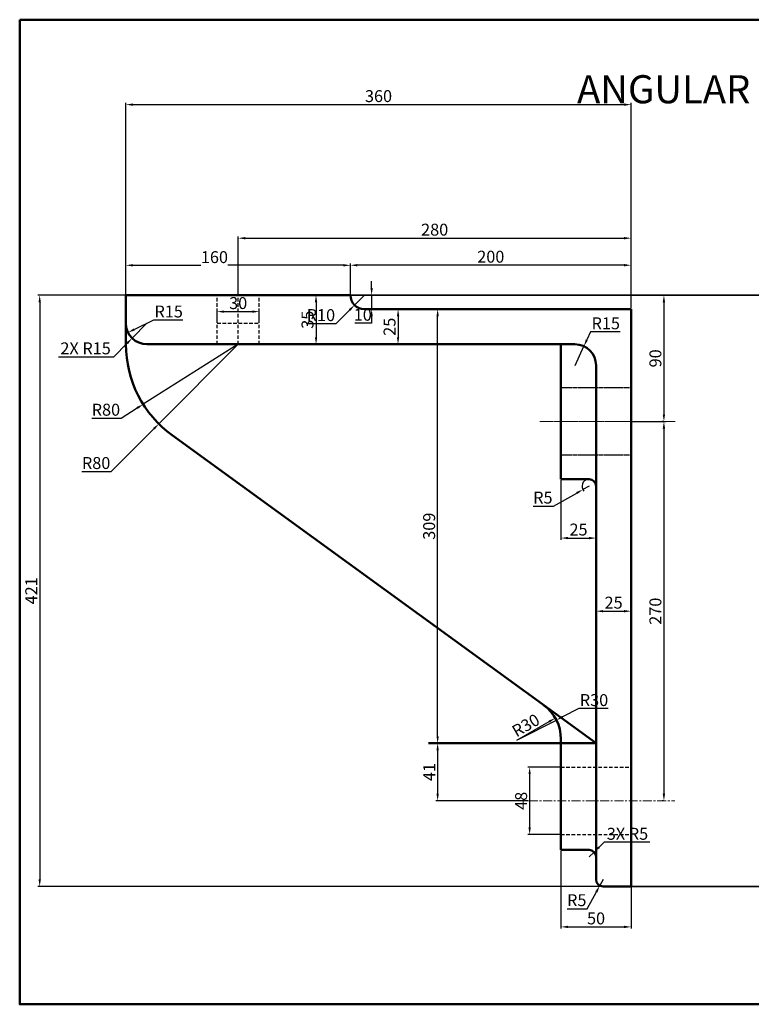
# Model space of a CAD drawing. Units: millimetres. Extents: x -624 to 605, y 670 to 1371.
# Tile 1 of 2: x -624 to -102, y 670 to 1371. Entities that reach past the tile are written whole.
import ezdxf

# ---------------------------------------------------------------- set-up
doc = ezdxf.new("R2010")
doc.units = ezdxf.units.MM
doc.header["$LTSCALE"] = 0.2
doc.linetypes.add('CENTER', pattern=[50.8, 31.75, -6.35, 6.35, -6.35])
doc.linetypes.add('DASHED', pattern=[19.05, 12.7, -6.35])
for name, color, linetype, lineweight in [('M-CNTR', 1, 'CENTER', 18), ('M-DIMS', 2, 'Continuous', 25), ('M-HIDN', 4, 'DASHED', 25), ('M-OUTL', 7, 'Continuous', 50), ('M-TEXT', 7, 'Continuous', 25)]:
    doc.layers.add(name, color=color, linetype=linetype, lineweight=lineweight)
doc.styles.get("Standard").update_dxf_attribs({"font": 'arial.ttf'})
doc.dimstyles.new('ISO-25', dxfattribs={"dimtxt": 8.5, "dimasz": 5, "dimexe": 1.25, "dimexo": 0.625, "dimtad": 1, "dimtoh": 1, "dimtxsty": 'Standard', "dimcen": 2.5, "dimadec": 0, "dimazin": 0, "dimtfac": 1, "dimtmove": 0, "dimatfit": 3, "dimfxl": 1, "dimarcsym": 0})

# ---------------------------------------------------------------- blocks, each defined once
blk = doc.blocks.new('*D1')
at = {"layer": 'Defpoints', "color": 0, "ltscale": 0.2, "transparency": 16777216}
for p in [(-354.19, 1164.58), (-354.19, 1139.58), (-354.19, 1139.58)]:
    blk.add_point(p, dxfattribs=at)
at = {"layer": 'M-DIMS', "color": 0, "lineweight": -2, "ltscale": 0.2, "transparency": 16777216}
for p, q in [((-354.82, 1164.58), (-355.44, 1164.58)), ((-354.19, 1159.58), (-354.19, 1144.58)), ((-354.82, 1139.58), (-355.44, 1139.58))]:
    blk.add_line(p, q, dxfattribs=at)
at = {"layer": 'M-DIMS', "color": 0, "ltscale": 0.2, "transparency": 16777216}
for points in [[(-355.03, 1159.58), (-353.36, 1159.58), (-354.19, 1164.58)], [(-355.03, 1144.58), (-353.36, 1144.58), (-354.19, 1139.58)]]:
    blk.add_solid(points, dxfattribs=at)
at = {"layer": 'M-DIMS', "color": 0, "ltscale": 0.2, "transparency": 16777216, "insert": (-359.16, 1152.08), "char_height": 8.5, "attachment_point": 5, "rotation": 90}
blk.add_mtext('25', dxfattribs=at)
blk = doc.blocks.new('*D2')
at = {"layer": 'Defpoints', "color": 0, "ltscale": 0.2, "transparency": 16777216}
for p in [(-548.12, 1195.84), (-548.12, 1174.58), (-388.12, 1174.58)]:
    blk.add_point(p, dxfattribs=at)
at = {"layer": 'M-DIMS', "color": 0, "lineweight": -2, "ltscale": 0.2, "transparency": 16777216}
for p, q in [((-548.12, 1175.21), (-548.12, 1197.09)), ((-543.12, 1195.84), (-494.63, 1195.84)), ((-393.12, 1195.84), (-475.43, 1195.84)), ((-388.12, 1175.21), (-388.12, 1197.09))]:
    blk.add_line(p, q, dxfattribs=at)
at = {"layer": 'M-DIMS', "color": 0, "ltscale": 0.2, "transparency": 16777216}
for points in [[(-543.12, 1196.68), (-543.12, 1195.01), (-548.12, 1195.84)], [(-393.12, 1196.68), (-393.12, 1195.01), (-388.12, 1195.84)]]:
    blk.add_solid(points, dxfattribs=at)
at = {"layer": 'M-DIMS', "color": 0, "ltscale": 0.2, "transparency": 16777216, "insert": (-485.03, 1200.55), "char_height": 8.5, "attachment_point": 5}
blk.add_mtext('160', dxfattribs=at)
blk = doc.blocks.new('*D3')
at = {"layer": 'Defpoints', "color": 0, "ltscale": 0.2, "transparency": 16777216}
for p in [(-388.12, 1174.58), (-373.46, 1164.58), (-373.03, 1164.58)]:
    blk.add_point(p, dxfattribs=at)
at = {"layer": 'M-DIMS', "color": 0, "lineweight": -2, "ltscale": 0.2, "transparency": 16777216}
for p, q in [((-373.03, 1179.58), (-373.03, 1184.58)), ((-387.5, 1174.58), (-371.78, 1174.58)), ((-373.03, 1174.58), (-373.03, 1164.58)), ((-372.83, 1164.58), (-371.78, 1164.58)), ((-373.03, 1159.58), (-373.03, 1154.58)), ((-373.03, 1154.58), (-385, 1154.58))]:
    blk.add_line(p, q, dxfattribs=at)
at = {"layer": 'M-DIMS', "color": 0, "ltscale": 0.2, "transparency": 16777216}
for points in [[(-373.87, 1179.58), (-372.2, 1179.58), (-373.03, 1174.58)], [(-373.87, 1159.58), (-372.2, 1159.58), (-373.03, 1164.58)]]:
    blk.add_solid(points, dxfattribs=at)
at = {"layer": 'M-DIMS', "color": 0, "ltscale": 0.2, "transparency": 16777216, "insert": (-379.33, 1159.55), "char_height": 8.5, "attachment_point": 5}
blk.add_mtext('10', dxfattribs=at)
blk = doc.blocks.new('*D4')
at = {"layer": 'Defpoints', "color": 0, "ltscale": 0.2, "transparency": 16777216}
for p in [(-388.12, 1195.89), (-388.12, 1174.58), (-188.12, 1164.58)]:
    blk.add_point(p, dxfattribs=at)
at = {"layer": 'M-DIMS', "color": 0, "lineweight": -2, "ltscale": 0.2, "transparency": 16777216}
for p, q in [((-388.12, 1175.21), (-388.12, 1197.14)), ((-193.12, 1195.89), (-383.12, 1195.89)), ((-188.12, 1165.21), (-188.12, 1197.14))]:
    blk.add_line(p, q, dxfattribs=at)
at = {"layer": 'M-DIMS', "color": 0, "ltscale": 0.2, "transparency": 16777216}
for points in [[(-383.12, 1196.73), (-383.12, 1195.06), (-388.12, 1195.89)], [(-193.12, 1196.73), (-193.12, 1195.06), (-188.12, 1195.89)]]:
    blk.add_solid(points, dxfattribs=at)
at = {"layer": 'M-DIMS', "color": 0, "ltscale": 0.2, "transparency": 16777216, "insert": (-288.12, 1200.86), "char_height": 8.5, "attachment_point": 5}
blk.add_mtext('200', dxfattribs=at)
blk = doc.blocks.new('*D5')
at = {"layer": 'Defpoints', "color": 0, "ltscale": 0.2, "transparency": 16777216}
for p in [(-453.12, 1162.86), (-483.12, 1154.58), (-453.12, 1154.58)]:
    blk.add_point(p, dxfattribs=at)
at = {"layer": 'M-DIMS', "color": 0, "lineweight": -2, "ltscale": 0.2, "transparency": 16777216}
for p, q in [((-483.12, 1155.21), (-483.12, 1164.11)), ((-453.12, 1155.21), (-453.12, 1164.11)), ((-478.12, 1162.86), (-458.12, 1162.86))]:
    blk.add_line(p, q, dxfattribs=at)
at = {"layer": 'M-DIMS', "color": 0, "ltscale": 0.2, "transparency": 16777216}
for points in [[(-478.12, 1163.69), (-478.12, 1162.03), (-483.12, 1162.86)], [(-458.12, 1163.69), (-458.12, 1162.03), (-453.12, 1162.86)]]:
    blk.add_solid(points, dxfattribs=at)
at = {"layer": 'M-DIMS', "color": 0, "ltscale": 0.2, "transparency": 16777216, "insert": (-468.12, 1167.83), "char_height": 8.5, "attachment_point": 5}
blk.add_mtext('30', dxfattribs=at)
blk = doc.blocks.new('*D6')
at = {"layer": 'Defpoints', "color": 0, "ltscale": 0.2, "transparency": 16777216}
for p in [(-410.05, 1174.58), (-412.64, 1139.58), (-410.05, 1139.58)]:
    blk.add_point(p, dxfattribs=at)
at = {"layer": 'M-DIMS', "color": 0, "lineweight": -2, "ltscale": 0.2, "transparency": 16777216}
for p, q in [((-410.68, 1174.58), (-413.89, 1174.58)), ((-412.64, 1169.58), (-412.64, 1144.58)), ((-410.68, 1139.58), (-413.89, 1139.58))]:
    blk.add_line(p, q, dxfattribs=at)
at = {"layer": 'M-DIMS', "color": 0, "ltscale": 0.2, "transparency": 16777216}
for points in [[(-413.47, 1169.58), (-411.81, 1169.58), (-412.64, 1174.58)], [(-413.47, 1144.58), (-411.81, 1144.58), (-412.64, 1139.58)]]:
    blk.add_solid(points, dxfattribs=at)
at = {"layer": 'M-DIMS', "color": 0, "ltscale": 0.2, "transparency": 16777216, "insert": (-417.61, 1157.08), "char_height": 8.5, "attachment_point": 5, "rotation": 90}
blk.add_mtext('35', dxfattribs=at)
blk = doc.blocks.new('*D7')
at = {"layer": 'Defpoints', "color": 0, "ltscale": 0.2, "transparency": 16777216}
for p in [(-188.12, 1215.14), (-468.12, 1174.58), (-188.12, 1164.58)]:
    blk.add_point(p, dxfattribs=at)
at = {"layer": 'M-DIMS', "color": 0, "lineweight": -2, "ltscale": 0.2, "transparency": 16777216}
for p, q in [((-468.12, 1175.21), (-468.12, 1216.39)), ((-463.12, 1215.14), (-193.12, 1215.14)), ((-188.12, 1165.21), (-188.12, 1216.39))]:
    blk.add_line(p, q, dxfattribs=at)
at = {"layer": 'M-DIMS', "color": 0, "ltscale": 0.2, "transparency": 16777216}
for points in [[(-463.12, 1215.97), (-463.12, 1214.31), (-468.12, 1215.14)], [(-193.12, 1215.97), (-193.12, 1214.31), (-188.12, 1215.14)]]:
    blk.add_solid(points, dxfattribs=at)
at = {"layer": 'M-DIMS', "color": 0, "ltscale": 0.2, "transparency": 16777216, "insert": (-328.12, 1220.11), "char_height": 8.5, "attachment_point": 5}
blk.add_mtext('280', dxfattribs=at)
blk = doc.blocks.new('*D8')
at = {"layer": 'Defpoints', "color": 0, "ltscale": 0.2, "transparency": 16777216}
for p in [(-533.12, 1154.58), (-546.59, 1147.98)]:
    blk.add_point(p, dxfattribs=at)
at = {"layer": 'M-DIMS', "color": 0, "lineweight": -2, "ltscale": 0.2, "transparency": 16777216}
for p, q in [((-528.44, 1156.87), (-542.1, 1150.18)), ((-507.44, 1156.87), (-528.44, 1156.87))]:
    blk.add_line(p, q, dxfattribs=at)
at = {"layer": 'M-DIMS', "color": 0, "ltscale": 0.2, "transparency": 16777216}
blk.add_solid([(-542.47, 1150.93), (-541.74, 1149.43), (-546.59, 1147.98)], dxfattribs=at)
at = {"layer": 'M-DIMS', "color": 0, "ltscale": 0.2, "transparency": 16777216, "insert": (-517.63, 1161.84), "char_height": 8.5, "attachment_point": 5}
blk.add_mtext('R15', dxfattribs=at)
blk = doc.blocks.new('*D9')
at = {"layer": 'Defpoints', "color": 0, "ltscale": 0.2, "transparency": 16777216}
for p in [(-468.12, 1139.58), (-535.79, 1096.91)]:
    blk.add_point(p, dxfattribs=at)
at = {"layer": 'M-DIMS', "color": 0, "lineweight": -2, "ltscale": 0.2, "transparency": 16777216}
for p, q in [((-468.12, 1139.58), (-535.79, 1096.91)), ((-551.59, 1086.95), (-540.02, 1094.24)), ((-572.5, 1086.95), (-551.59, 1086.95))]:
    blk.add_line(p, q, dxfattribs=at)
at = {"layer": 'M-DIMS', "color": 0, "ltscale": 0.2, "transparency": 16777216}
blk.add_solid([(-540.47, 1094.95), (-539.58, 1093.54), (-535.79, 1096.91)], dxfattribs=at)
at = {"layer": 'M-DIMS', "color": 0, "ltscale": 0.2, "transparency": 16777216, "insert": (-562.36, 1091.91), "char_height": 8.5, "attachment_point": 5}
blk.add_mtext('R80', dxfattribs=at)
blk = doc.blocks.new('*D10')
at = {"layer": 'Defpoints', "color": 0, "ltscale": 0.2, "transparency": 16777216}
for p in [(-326.01, 1164.58), (-305.32, 1164.58), (-305.32, 855.58)]:
    blk.add_point(p, dxfattribs=at)
at = {"layer": 'M-DIMS', "color": 0, "lineweight": -2, "ltscale": 0.2, "transparency": 16777216}
for p, q in [((-305.94, 1164.58), (-327.26, 1164.58)), ((-326.01, 860.58), (-326.01, 1159.58)), ((-305.94, 855.58), (-327.26, 855.58))]:
    blk.add_line(p, q, dxfattribs=at)
at = {"layer": 'M-DIMS', "color": 0, "ltscale": 0.2, "transparency": 16777216}
for points in [[(-326.84, 1159.58), (-325.17, 1159.58), (-326.01, 1164.58)], [(-326.84, 860.58), (-325.17, 860.58), (-326.01, 855.58)]]:
    blk.add_solid(points, dxfattribs=at)
at = {"layer": 'M-DIMS', "color": 0, "ltscale": 0.2, "transparency": 16777216, "insert": (-330.97, 1010.08), "char_height": 8.5, "attachment_point": 5, "rotation": 90}
blk.add_mtext('309', dxfattribs=at)
blk = doc.blocks.new('*D11')
at = {"layer": 'Defpoints', "color": 0, "ltscale": 0.2, "transparency": 16777216}
for p in [(-316.6, 855.58), (-326.01, 814.58), (-260.98, 814.58)]:
    blk.add_point(p, dxfattribs=at)
at = {"layer": 'M-DIMS', "color": 0, "lineweight": -2, "ltscale": 0.2, "transparency": 16777216}
for p, q in [((-317.22, 855.58), (-327.26, 855.58)), ((-326.01, 850.58), (-326.01, 819.58)), ((-261.61, 814.58), (-327.26, 814.58))]:
    blk.add_line(p, q, dxfattribs=at)
at = {"layer": 'M-DIMS', "color": 0, "ltscale": 0.2, "transparency": 16777216}
for points in [[(-326.84, 850.58), (-325.17, 850.58), (-326.01, 855.58)], [(-326.84, 819.58), (-325.17, 819.58), (-326.01, 814.58)]]:
    blk.add_solid(points, dxfattribs=at)
at = {"layer": 'M-DIMS', "color": 0, "ltscale": 0.2, "transparency": 16777216, "insert": (-330.9, 835.08), "char_height": 8.5, "attachment_point": 5, "rotation": 90}
blk.add_mtext('41', dxfattribs=at)
blk = doc.blocks.new('*D12')
at = {"layer": 'Defpoints', "color": 0, "ltscale": 0.2, "transparency": 16777216}
for p in [(-238.12, 838.58), (-260.44, 790.58), (-238.12, 790.58)]:
    blk.add_point(p, dxfattribs=at)
at = {"layer": 'M-DIMS', "color": 0, "lineweight": -2, "ltscale": 0.2, "transparency": 16777216}
for p, q in [((-238.75, 838.58), (-261.69, 838.58)), ((-260.44, 833.58), (-260.44, 795.58)), ((-238.75, 790.58), (-261.69, 790.58))]:
    blk.add_line(p, q, dxfattribs=at)
at = {"layer": 'M-DIMS', "color": 0, "ltscale": 0.2, "transparency": 16777216}
for points in [[(-261.28, 833.58), (-259.61, 833.58), (-260.44, 838.58)], [(-261.28, 795.58), (-259.61, 795.58), (-260.44, 790.58)]]:
    blk.add_solid(points, dxfattribs=at)
at = {"layer": 'M-DIMS', "color": 0, "ltscale": 0.2, "transparency": 16777216, "insert": (-265.41, 814.58), "char_height": 8.5, "attachment_point": 5, "rotation": 90}
blk.add_mtext('48', dxfattribs=at)
blk = doc.blocks.new('*D13')
at = {"layer": 'Defpoints', "color": 0, "ltscale": 0.2, "transparency": 16777216}
for p in [(-242.17, 873.48), (-268.12, 858.44)]:
    blk.add_point(p, dxfattribs=at)
at = {"layer": 'M-DIMS', "color": 0, "lineweight": -2, "ltscale": 0.2, "transparency": 16777216}
blk.add_line((-269.45, 857.67), (-246.49, 870.97), dxfattribs=at)
at = {"layer": 'M-DIMS', "color": 0, "ltscale": 0.2, "transparency": 16777216}
blk.add_solid([(-246.91, 871.7), (-246.08, 870.25), (-242.17, 873.48)], dxfattribs=at)
at = {"layer": 'M-DIMS', "color": 0, "ltscale": 0.2, "transparency": 16777216, "insert": (-262.63, 867.37), "char_height": 8.5, "attachment_point": 5, "rotation": 30.09395}
blk.add_mtext('R30', dxfattribs=at)
blk = doc.blocks.new('*D14')
at = {"layer": 'Defpoints', "color": 0, "ltscale": 0.2, "transparency": 16777216}
for p in [(-238.12, 779.58), (-188.12, 779.58), (-188.12, 724.81)]:
    blk.add_point(p, dxfattribs=at)
at = {"layer": 'M-DIMS', "color": 0, "lineweight": -2, "ltscale": 0.2, "transparency": 16777216}
for p, q in [((-238.12, 778.96), (-238.12, 723.56)), ((-188.12, 778.96), (-188.12, 723.56)), ((-233.12, 724.81), (-193.12, 724.81))]:
    blk.add_line(p, q, dxfattribs=at)
at = {"layer": 'M-DIMS', "color": 0, "ltscale": 0.2, "transparency": 16777216}
for points in [[(-233.12, 725.64), (-233.12, 723.97), (-238.12, 724.81)], [(-193.12, 725.64), (-193.12, 723.97), (-188.12, 724.81)]]:
    blk.add_solid(points, dxfattribs=at)
at = {"layer": 'M-DIMS', "color": 0, "ltscale": 0.2, "transparency": 16777216, "insert": (-213.12, 729.77), "char_height": 8.5, "attachment_point": 5}
blk.add_mtext('50', dxfattribs=at)
blk = doc.blocks.new('*D15')
at = {"layer": 'Defpoints', "color": 0, "ltscale": 0.2, "transparency": 16777216}
for p in [(-208.12, 758.58), (-210.5, 754.18)]:
    blk.add_point(p, dxfattribs=at)
at = {"layer": 'M-DIMS', "color": 0, "lineweight": -2, "ltscale": 0.2, "transparency": 16777216}
for p, q in [((-208.12, 758.58), (-210.5, 754.18)), ((-219.36, 737.77), (-212.88, 749.78)), ((-233.75, 737.77), (-219.36, 737.77))]:
    blk.add_line(p, q, dxfattribs=at)
at = {"layer": 'M-DIMS', "color": 0, "ltscale": 0.2, "transparency": 16777216}
blk.add_solid([(-213.61, 750.18), (-212.14, 749.39), (-210.5, 754.18)], dxfattribs=at)
at = {"layer": 'M-DIMS', "color": 0, "ltscale": 0.2, "transparency": 16777216, "insert": (-226.87, 742.72), "char_height": 8.5, "attachment_point": 5}
blk.add_mtext('R5', dxfattribs=at)
blk = doc.blocks.new('*D16')
at = {"layer": 'Defpoints', "color": 0, "ltscale": 0.2, "transparency": 16777216}
for p in [(-213.12, 949.58), (-188.12, 949.58), (-188.12, 949.58)]:
    blk.add_point(p, dxfattribs=at)
at = {"layer": 'M-DIMS', "color": 0, "lineweight": -2, "ltscale": 0.2, "transparency": 16777216}
for p, q in [((-213.12, 950.21), (-213.12, 950.83)), ((-208.12, 949.58), (-193.12, 949.58)), ((-188.12, 950.21), (-188.12, 950.83))]:
    blk.add_line(p, q, dxfattribs=at)
at = {"layer": 'M-DIMS', "color": 0, "ltscale": 0.2, "transparency": 16777216}
for points in [[(-208.12, 950.41), (-208.12, 948.75), (-213.12, 949.58)], [(-193.12, 950.41), (-193.12, 948.75), (-188.12, 949.58)]]:
    blk.add_solid(points, dxfattribs=at)
at = {"layer": 'M-DIMS', "color": 0, "ltscale": 0.2, "transparency": 16777216, "insert": (-200.62, 954.55), "char_height": 8.5, "attachment_point": 5}
blk.add_mtext('25', dxfattribs=at)
blk = doc.blocks.new('*D17')
at = {"layer": 'Defpoints', "color": 0, "ltscale": 0.2, "transparency": 16777216}
for p in [(-388.12, 1174.58), (-188.12, 1084.58), (-164.76, 1084.58)]:
    blk.add_point(p, dxfattribs=at)
at = {"layer": 'M-DIMS', "color": 0, "lineweight": -2, "ltscale": 0.2, "transparency": 16777216}
for p, q in [((-387.5, 1174.58), (-163.51, 1174.58)), ((-164.76, 1169.58), (-164.76, 1089.58)), ((-187.5, 1084.58), (-163.51, 1084.58))]:
    blk.add_line(p, q, dxfattribs=at)
at = {"layer": 'M-DIMS', "color": 0, "ltscale": 0.2, "transparency": 16777216}
for points in [[(-165.6, 1169.58), (-163.93, 1169.58), (-164.76, 1174.58)], [(-165.6, 1089.58), (-163.93, 1089.58), (-164.76, 1084.58)]]:
    blk.add_solid(points, dxfattribs=at)
at = {"layer": 'M-DIMS', "color": 0, "ltscale": 0.2, "transparency": 16777216, "insert": (-169.73, 1129.58), "char_height": 8.5, "attachment_point": 5, "rotation": 90}
blk.add_mtext('90', dxfattribs=at)
blk = doc.blocks.new('*D18')
at = {"layer": 'Defpoints', "color": 0, "ltscale": 0.2, "transparency": 16777216}
for p in [(-164.76, 1084.58), (-164.76, 814.58), (-164.76, 814.58)]:
    blk.add_point(p, dxfattribs=at)
at = {"layer": 'M-DIMS', "color": 0, "lineweight": -2, "ltscale": 0.2, "transparency": 16777216}
for p, q in [((-165.39, 1084.58), (-166.01, 1084.58)), ((-164.76, 1079.58), (-164.76, 819.58)), ((-165.39, 814.58), (-166.01, 814.58))]:
    blk.add_line(p, q, dxfattribs=at)
at = {"layer": 'M-DIMS', "color": 0, "ltscale": 0.2, "transparency": 16777216}
for points in [[(-165.6, 1079.58), (-163.93, 1079.58), (-164.76, 1084.58)], [(-165.6, 819.58), (-163.93, 819.58), (-164.76, 814.58)]]:
    blk.add_solid(points, dxfattribs=at)
at = {"layer": 'M-DIMS', "color": 0, "ltscale": 0.2, "transparency": 16777216, "insert": (-169.73, 949.58), "char_height": 8.5, "attachment_point": 5, "rotation": 90}
blk.add_mtext('270', dxfattribs=at)
blk = doc.blocks.new('*D19')
at = {"layer": 'Defpoints', "color": 0, "ltscale": 0.2, "transparency": 16777216}
for p in [(-238.12, 1043.58), (-213.12, 1043.58), (-213.12, 1001.63)]:
    blk.add_point(p, dxfattribs=at)
at = {"layer": 'M-DIMS', "color": 0, "lineweight": -2, "ltscale": 0.2, "transparency": 16777216}
for p, q in [((-238.12, 1042.96), (-238.12, 1000.38)), ((-213.12, 1042.96), (-213.12, 1000.38)), ((-233.12, 1001.63), (-218.12, 1001.63))]:
    blk.add_line(p, q, dxfattribs=at)
at = {"layer": 'M-DIMS', "color": 0, "ltscale": 0.2, "transparency": 16777216}
for points in [[(-233.12, 1002.47), (-233.12, 1000.8), (-238.12, 1001.63)], [(-218.12, 1002.47), (-218.12, 1000.8), (-213.12, 1001.63)]]:
    blk.add_solid(points, dxfattribs=at)
at = {"layer": 'M-DIMS', "color": 0, "ltscale": 0.2, "transparency": 16777216, "insert": (-225.62, 1006.6), "char_height": 8.5, "attachment_point": 5}
blk.add_mtext('25', dxfattribs=at)
blk = doc.blocks.new('*D20')
at = {"layer": 'Defpoints', "color": 0, "ltscale": 0.2, "transparency": 16777216}
for p in [(-218.12, 1038.58), (-222.49, 1036.14)]:
    blk.add_point(p, dxfattribs=at)
at = {"layer": 'M-DIMS', "color": 0, "lineweight": -2, "ltscale": 0.2, "transparency": 16777216}
for p, q in [((-218.12, 1038.58), (-222.49, 1036.14)), ((-243.51, 1024.41), (-226.86, 1033.71)), ((-257.9, 1024.41), (-243.51, 1024.41))]:
    blk.add_line(p, q, dxfattribs=at)
blk.add_arc((-218.12, 1038.58), 5, 97.16197, 223.49709, dxfattribs=at)
at = {"layer": 'M-DIMS', "color": 0, "ltscale": 0.2, "transparency": 16777216}
blk.add_solid([(-227.26, 1034.43), (-226.45, 1032.98), (-222.49, 1036.14)], dxfattribs=at)
at = {"layer": 'M-DIMS', "color": 0, "ltscale": 0.2, "transparency": 16777216, "insert": (-251.02, 1029.36), "char_height": 8.5, "attachment_point": 5}
blk.add_mtext('R5', dxfattribs=at)
blk = doc.blocks.new('*D21')
at = {"layer": 'Defpoints', "color": 0, "ltscale": 0.2, "transparency": 16777216}
for p in [(-221.8, 1138.18), (-228.12, 1124.58)]:
    blk.add_point(p, dxfattribs=at)
at = {"layer": 'M-DIMS', "color": 0, "lineweight": -2, "ltscale": 0.2, "transparency": 16777216}
for p, q in [((-217.02, 1148.47), (-219.69, 1142.72)), ((-196.02, 1148.47), (-217.02, 1148.47)), ((-228.12, 1124.58), (-221.8, 1138.18))]:
    blk.add_line(p, q, dxfattribs=at)
at = {"layer": 'M-DIMS', "color": 0, "ltscale": 0.2, "transparency": 16777216}
blk.add_solid([(-220.45, 1143.07), (-218.94, 1142.37), (-221.8, 1138.18)], dxfattribs=at)
at = {"layer": 'M-DIMS', "color": 0, "ltscale": 0.2, "transparency": 16777216, "insert": (-206.21, 1153.43), "char_height": 8.5, "attachment_point": 5}
blk.add_mtext('R15', dxfattribs=at)
blk = doc.blocks.new('*D46')
at = {"layer": 'Defpoints', "color": 0, "ltscale": 0.2, "transparency": 16777216}
for p in [(-188.12, 1310.22), (-548.12, 1174.58), (-188.12, 1164.58)]:
    blk.add_point(p, dxfattribs=at)
at = {"layer": 'M-DIMS', "color": 0, "lineweight": -2, "ltscale": 0.2, "transparency": 16777216}
for p, q in [((-548.12, 1175.21), (-548.12, 1311.47)), ((-188.12, 1165.21), (-188.12, 1311.47)), ((-543.12, 1310.22), (-193.12, 1310.22))]:
    blk.add_line(p, q, dxfattribs=at)
at = {"layer": 'M-DIMS', "color": 0, "ltscale": 0.2, "transparency": 16777216}
for points in [[(-543.12, 1311.05), (-543.12, 1309.39), (-548.12, 1310.22)], [(-193.12, 1311.05), (-193.12, 1309.39), (-188.12, 1310.22)]]:
    blk.add_solid(points, dxfattribs=at)
at = {"layer": 'M-DIMS', "color": 0, "ltscale": 0.2, "transparency": 16777216, "insert": (-368.12, 1315.19), "char_height": 8.5, "attachment_point": 5}
blk.add_mtext('360', dxfattribs=at)
blk = doc.blocks.new('*D47')
at = {"layer": 'Defpoints', "color": 0, "ltscale": 0.2, "transparency": 16777216}
for p in [(-548.12, 1174.58), (-188.12, 753.58), (516.74, 753.58)]:
    blk.add_point(p, dxfattribs=at)
at = {"layer": 'M-DIMS', "color": 0, "lineweight": -2, "ltscale": 0.2, "transparency": 16777216}
for p, q in [((-547.5, 1174.58), (517.99, 1174.58)), ((516.74, 1169.58), (516.74, 758.58)), ((-187.5, 753.58), (517.99, 753.58))]:
    blk.add_line(p, q, dxfattribs=at)
at = {"layer": 'M-DIMS', "color": 0, "ltscale": 0.2, "transparency": 16777216}
for points in [[(515.9, 1169.58), (517.57, 1169.58), (516.74, 1174.58)], [(515.9, 758.58), (517.57, 758.58), (516.74, 753.58)]]:
    blk.add_solid(points, dxfattribs=at)
at = {"layer": 'M-DIMS', "color": 0, "ltscale": 0.2, "transparency": 16777216, "insert": (511.84, 964.08), "char_height": 8.5, "attachment_point": 5, "rotation": 90}
blk.add_mtext('421', dxfattribs=at)
blk = doc.blocks.new('*D48')
at = {"layer": 'Defpoints', "color": 0, "ltscale": 0.2, "transparency": 16777216}
for p in [(-34.68, 1174.58), (-609.54, 753.58), (210.32, 753.58)]:
    blk.add_point(p, dxfattribs=at)
at = {"layer": 'M-DIMS', "color": 0, "lineweight": -2, "ltscale": 0.2, "transparency": 16777216}
for p, q in [((-35.3, 1174.58), (-610.79, 1174.58)), ((-609.54, 1169.58), (-609.54, 758.58)), ((209.7, 753.58), (-610.79, 753.58))]:
    blk.add_line(p, q, dxfattribs=at)
at = {"layer": 'M-DIMS', "color": 0, "ltscale": 0.2, "transparency": 16777216}
for points in [[(-610.37, 1169.58), (-608.71, 1169.58), (-609.54, 1174.58)], [(-610.37, 758.58), (-608.71, 758.58), (-609.54, 753.58)]]:
    blk.add_solid(points, dxfattribs=at)
at = {"layer": 'M-DIMS', "color": 0, "ltscale": 0.2, "transparency": 16777216, "insert": (-614.43, 964.08), "char_height": 8.5, "attachment_point": 5, "rotation": 90}
blk.add_mtext('421', dxfattribs=at)
blk = doc.blocks.new('*D49')
at = {"layer": 'Defpoints', "color": 0, "ltscale": 0.2, "transparency": 16777216}
for p in [(-468.12, 1139.58), (-524.64, 1082.96)]:
    blk.add_point(p, dxfattribs=at)
at = {"layer": 'M-DIMS', "color": 0, "lineweight": -2, "ltscale": 0.2, "transparency": 16777216}
for p, q in [((-468.12, 1139.58), (-524.64, 1082.96)), ((-558.55, 1048.99), (-528.17, 1079.42)), ((-579.46, 1048.99), (-558.55, 1048.99))]:
    blk.add_line(p, q, dxfattribs=at)
at = {"layer": 'M-DIMS', "color": 0, "ltscale": 0.2, "transparency": 16777216}
blk.add_solid([(-528.76, 1080.01), (-527.58, 1078.83), (-524.64, 1082.96)], dxfattribs=at)
at = {"layer": 'M-DIMS', "color": 0, "ltscale": 0.2, "transparency": 16777216, "insert": (-569.32, 1053.95), "char_height": 8.5, "attachment_point": 5}
blk.add_mtext('R80', dxfattribs=at)
blk = doc.blocks.new('*D50')
at = {"layer": 'Defpoints', "color": 0, "ltscale": 0.2, "transparency": 16777216}
for p in [(-241.4, 872.06), (-268.12, 858.44)]:
    blk.add_point(p, dxfattribs=at)
at = {"layer": 'M-DIMS', "color": 0, "lineweight": -2, "ltscale": 0.2, "transparency": 16777216}
for p, q in [((-225.36, 880.24), (-236.94, 874.33)), ((-204.45, 880.24), (-225.36, 880.24)), ((-268.12, 858.44), (-241.4, 872.06))]:
    blk.add_line(p, q, dxfattribs=at)
at = {"layer": 'M-DIMS', "color": 0, "ltscale": 0.2, "transparency": 16777216}
blk.add_solid([(-237.32, 875.08), (-236.56, 873.59), (-241.4, 872.06)], dxfattribs=at)
at = {"layer": 'M-DIMS', "color": 0, "ltscale": 0.2, "transparency": 16777216, "insert": (-214.59, 885.2), "char_height": 8.5, "attachment_point": 5}
blk.add_mtext('R30', dxfattribs=at)
blk = doc.blocks.new('*D51')
at = {"layer": 'Defpoints', "color": 0, "ltscale": 0.2, "transparency": 16777216}
for p in [(-533.12, 1154.58), (-543.68, 1143.92)]:
    blk.add_point(p, dxfattribs=at)
at = {"layer": 'M-DIMS', "color": 0, "lineweight": -2, "ltscale": 0.2, "transparency": 16777216}
for p, q in [((-533.12, 1154.58), (-543.68, 1143.92)), ((-556.82, 1130.65), (-547.2, 1140.37)), ((-596.23, 1130.65), (-556.82, 1130.65))]:
    blk.add_line(p, q, dxfattribs=at)
at = {"layer": 'M-DIMS', "color": 0, "ltscale": 0.2, "transparency": 16777216}
blk.add_solid([(-547.79, 1140.95), (-546.6, 1139.78), (-543.68, 1143.92)], dxfattribs=at)
at = {"layer": 'M-DIMS', "color": 0, "ltscale": 0.2, "transparency": 16777216, "insert": (-576.84, 1135.61), "char_height": 8.5, "attachment_point": 5}
blk.add_mtext('2X R15', dxfattribs=at)
blk = doc.blocks.new('*D52')
at = {"layer": 'Defpoints', "color": 0, "ltscale": 0.2, "transparency": 16777216}
for p in [(-218.12, 774.58), (-214.54, 778.06)]:
    blk.add_point(p, dxfattribs=at)
at = {"layer": 'M-DIMS', "color": 0, "lineweight": -2, "ltscale": 0.2, "transparency": 16777216}
for p, q in [((-207.36, 785.03), (-210.95, 781.55)), ((-174.71, 785.03), (-207.36, 785.03)), ((-218.12, 774.58), (-214.54, 778.06))]:
    blk.add_line(p, q, dxfattribs=at)
at = {"layer": 'M-DIMS', "color": 0, "ltscale": 0.2, "transparency": 16777216}
blk.add_solid([(-211.53, 782.15), (-210.37, 780.95), (-214.54, 778.06)], dxfattribs=at)
at = {"layer": 'M-DIMS', "color": 0, "ltscale": 0.2, "transparency": 16777216, "insert": (-190.72, 790), "char_height": 8.5, "attachment_point": 5}
blk.add_mtext('3X R5', dxfattribs=at)
blk = doc.blocks.new('*D53')
at = {"layer": 'Defpoints', "color": 0, "ltscale": 0.2, "transparency": 16777216}
for p in [(-378.12, 1174.58), (-385.19, 1167.51)]:
    blk.add_point(p, dxfattribs=at)
at = {"layer": 'M-DIMS', "color": 0, "lineweight": -2, "ltscale": 0.2, "transparency": 16777216}
for p, q in [((-378.12, 1174.58), (-385.19, 1167.51)), ((-398.4, 1154.29), (-388.73, 1163.97)), ((-419.3, 1154.29), (-398.4, 1154.29))]:
    blk.add_line(p, q, dxfattribs=at)
at = {"layer": 'M-DIMS', "color": 0, "ltscale": 0.2, "transparency": 16777216}
blk.add_solid([(-389.32, 1164.56), (-388.14, 1163.38), (-385.19, 1167.51)], dxfattribs=at)
at = {"layer": 'M-DIMS', "color": 0, "ltscale": 0.2, "transparency": 16777216, "insert": (-409.16, 1159.26), "char_height": 8.5, "attachment_point": 5}
blk.add_mtext('R10', dxfattribs=at)

msp = doc.modelspace()

# ---------------------------------------------------------------- linework, layer by layer
at = {"layer": 'M-CNTR', "ltscale": 0.2}
msp.add_line((-253.198, 1084.58), (-156.652, 1084.58), dxfattribs=at)
at = {"layer": 'M-CNTR'}
msp.add_line((-260.98, 814.58), (-157.062, 814.58), dxfattribs=at)
at = {"layer": 'M-HIDN'}
for p, q in [((-483.124, 1139.58), (-483.124, 1174.58)), ((-468.124, 1139.58), (-468.124, 1174.58)), ((-453.124, 1139.58), (-453.124, 1174.58)), ((-483.124, 1154.58), (-453.124, 1154.58)), ((-238.124, 838.58), (-188.124, 838.58)), ((-238.124, 790.58), (-188.124, 790.58))]:
    msp.add_line(p, q, dxfattribs=at)
at = {"layer": 'M-HIDN', "ltscale": 0.2}
for p, q in [((-188.124, 1108.58), (-238.124, 1108.58)), ((-188.124, 1060.58), (-238.124, 1060.58))]:
    msp.add_line(p, q, dxfattribs=at)
at = {"layer": 'M-OUTL'}
for p, q in [((-388.124, 1174.58), (-548.124, 1174.58)), ((-548.124, 1174.58), (-548.124, 1154.58)), ((-388.124, 1174.58), (-388.124, 1174.58)), ((-378.124, 1164.58), (-188.124, 1164.58)), ((-188.124, 1164.58), (-188.124, 753.58)), ((-533.124, 1139.58), (-228.124, 1139.58)), ((-213.124, 774.58), (-213.124, 1124.58)), ((-213.124, 758.58), (-213.124, 774.58)), ((-188.124, 753.58), (-208.124, 753.58))]:
    msp.add_line(p, q, dxfattribs=at)
at = {"layer": 'M-OUTL', "ltscale": 0.2}
for p, q in [((-548.124, 1174.58), (-548.124, 1139.58)), ((-238.124, 1043.58), (-238.124, 1139.58)), ((-213.124, 855.58), (-515.125, 1074.843)), ((-218.124, 1043.58), (-238.124, 1043.58)), ((-332.616, 855.58), (-213.124, 855.58)), ((-238.124, 779.58), (-238.124, 858.439)), ((-218.124, 779.58), (-238.124, 779.58)), ((-188.124, 753.58), (-208.124, 753.58))]:
    msp.add_line(p, q, dxfattribs=at)
msp.add_lwpolyline([(-623.802, 1370.695), (604.533, 1370.695), (604.533, 669.699), (-623.802, 669.699)], close=True, dxfattribs=at)
at = {"layer": 'M-OUTL'}
for centre, radius, start, end in [((-378.124, 1174.58), 10, 180, 270), ((-533.124, 1154.58), 15, 180, 270), ((-228.124, 1124.58), 15, 0, 90), ((-218.124, 1038.58), 5, 0, 90), ((-218.124, 774.58), 5, 360, 90), ((-208.124, 758.58), 5, 180, 270)]:
    msp.add_arc(centre, radius, start, end, dxfattribs=at)
at = {"layer": 'M-OUTL', "ltscale": 0.2}
for centre, radius, start, end in [((-468.124, 1139.58), 80, 180, 234.0191), ((-268.124, 858.439), 30, 0, 54.0191)]:
    msp.add_arc(centre, radius, start, end, dxfattribs=at)

# ---------------------------------------------------------------- texts
at = {"layer": 'M-TEXT', "ltscale": 0.2, "insert": (-226.692, 1331.188), "char_height": 20, "attachment_point": 1}
msp.add_mtext_dynamic_manual_height_columns('ANGULAR CANTILEVER BRACKET', width=461.44309, gutter_width=12.5, heights=[0], dxfattribs=at)

# ---------------------------------------------------------------- dimensions: what is measured, and where the dimension line sits
at = {"layer": 'M-DIMS', "ltscale": 0.2}
for base, p1, p2, override, picture, middle in [((-188.124, 1310.221), (-548.124, 1174.58), (-188.124, 1164.58), {"dimdec": 0, "dimlfac": 1, "dimrnd": 0, "dimzin": 0, "dimdsep": 46, "dimlunit": 2}, '*D46', (-368.124, 1315.188)), ((-188.124, 1215.141), (-468.124, 1174.58), (-188.124, 1164.58), {"dimclrd": 0, "dimclre": 0, "dimclrt": 0}, '*D7', (-328.124, 1220.106)), ((-388.124, 1195.892), (-188.124, 1164.58), (-388.124, 1174.58), {"dimclrd": 0, "dimclre": 0, "dimclrt": 0}, '*D4', (-288.124, 1200.857)), ((-453.124, 1162.859), (-483.124, 1154.58), (-453.124, 1154.58), {"dimclrd": 0, "dimclre": 0, "dimclrt": 0}, '*D5', (-468.124, 1167.827)), ((-188.124, 949.58), (-213.124, 949.58), (-188.124, 949.58), {"dimclrd": 0, "dimclre": 0, "dimclrt": 0}, '*D16', (-200.624, 954.545)), ((-188.124, 724.805), (-238.124, 779.58), (-188.124, 779.58), {"dimclrd": 0, "dimclre": 0, "dimclrt": 0}, '*D14', (-213.124, 729.77))]:
    dim = msp.add_linear_dim(base=base, p1=p1, p2=p2, dimstyle='ISO-25', override=override, dxfattribs=at)
    dim.commit()
    dim.dimension.update_dxf_attribs({"geometry": picture, "text_midpoint": middle})
for base, p1, p2, override, picture, middle in [((-548.124, 1195.842), (-388.124, 1174.58), (-548.124, 1174.58), {"dimclrd": 0, "dimclre": 0, "dimclrt": 0, "dimtmove": 2}, '*D2', (-485.032, 1200.552)), ((-213.124, 1001.634), (-238.124, 1043.58), (-213.124, 1043.58), {"dimclrd": 0, "dimclre": 0, "dimclrt": 0}, '*D19', (-225.624, 1001.634))]:
    dim = msp.add_linear_dim(base=base, p1=p1, p2=p2, dimstyle='ISO-25', override=override, dxfattribs=at)
    dim.commit()
    dim.dimension.update_dxf_attribs({"geometry": picture, "text_midpoint": middle, "dimtype": 160})
for base, p1, p2, override, picture, middle in [((-373.032, 1164.58), (-388.124, 1174.58), (-373.455, 1164.58), {"dimclrd": 0, "dimclre": 0, "dimclrt": 0}, '*D3', (-379.33, 1159.545)), ((-609.541, 753.58), (-34.679, 1174.58), (210.321, 753.58), {"dimdec": 0, "dimlfac": 1, "dimrnd": 0, "dimzin": 0, "dimdsep": 46, "dimlunit": 2}, '*D48', (-614.433, 964.08)), ((516.737, 753.58), (-548.124, 1174.58), (-188.124, 753.58), {"dimdec": 0, "dimlfac": 1, "dimrnd": 0, "dimzin": 0, "dimdsep": 46, "dimlunit": 2}, '*D47', (511.845, 964.08)), ((-412.638, 1139.58), (-410.051, 1174.58), (-410.051, 1139.58), {"dimclrd": 0, "dimclre": 0, "dimclrt": 0}, '*D6', (-417.606, 1157.08)), ((-164.765, 1084.58), (-388.124, 1174.58), (-188.124, 1084.58), {"dimclrd": 0, "dimclre": 0, "dimclrt": 0}, '*D17', (-169.73, 1129.58)), ((-354.193, 1139.58), (-354.193, 1164.58), (-354.193, 1139.58), {"dimclrd": 0, "dimclre": 0, "dimclrt": 0}, '*D1', (-359.158, 1152.08)), ((-326.007, 1164.58), (-305.316, 855.58), (-305.316, 1164.58), {"dimclrd": 0, "dimclre": 0, "dimclrt": 0}, '*D10', (-330.974, 1010.08)), ((-164.765, 814.58), (-164.765, 1084.58), (-164.765, 814.58), {"dimclrd": 0, "dimclre": 0, "dimclrt": 0}, '*D18', (-169.73, 949.58)), ((-326.007, 814.58), (-316.599, 855.58), (-260.98, 814.58), {"dimclrd": 0, "dimclre": 0, "dimclrt": 0}, '*D11', (-330.899, 835.08)), ((-260.442, 790.58), (-238.124, 838.58), (-238.124, 790.58), {"dimclrd": 0, "dimclre": 0, "dimclrt": 0}, '*D12', (-265.407, 814.58))]:
    dim = msp.add_linear_dim(base=base, p1=p1, p2=p2, angle=90, dimstyle='ISO-25', override=override, dxfattribs=at)
    dim.commit()
    dim.dimension.update_dxf_attribs({"geometry": picture, "text_midpoint": middle})
for center, mpoint, override, picture, middle in [((-378.124, 1174.58), (-385.193, 1167.507), {"dimdec": 0, "dimlfac": 1, "dimrnd": 0, "dimzin": 0, "dimdsep": 46, "dimlunit": 2}, '*D53', (-409.163, 1159.259)), ((-468.124, 1139.58), (-535.793, 1096.909), {"dimclrd": 0, "dimclre": 0, "dimclrt": 0}, '*D9', (-562.36, 1091.91)), ((-208.124, 758.58), (-210.5, 754.181), {"dimclrd": 0, "dimclre": 0, "dimclrt": 0}, '*D15', (-226.869, 742.722))]:
    dim = msp.add_radius_dim(center=center, mpoint=mpoint, dimstyle='ISO-25', override=override, dxfattribs=at)
    dim.commit()
    dim.dimension.update_dxf_attribs({"geometry": picture, "text_midpoint": middle})
for center, mpoint, override, picture, middle in [((-533.124, 1154.58), (-546.595, 1147.982), {"dimclrd": 0, "dimclre": 0, "dimclrt": 0}, '*D8', (-517.63, 1156.873)), ((-228.124, 1124.58), (-221.801, 1138.182), {"dimclrd": 0, "dimclre": 0, "dimclrt": 0}, '*D21', (-206.209, 1148.466)), ((-468.124, 1139.58), (-524.64, 1082.96), {"dimdec": 0, "dimlfac": 1, "dimrnd": 0, "dimzin": 0, "dimdsep": 46, "dimlunit": 2}, '*D49', (-569.316, 1048.987)), ((-218.124, 1038.58), (-222.49, 1036.143), {"dimclrd": 0, "dimclre": 0, "dimclrt": 0}, '*D20', (-251.02, 1024.408)), ((-268.124, 858.439), (-241.396, 872.062), {"dimdec": 0, "dimlfac": 1, "dimrnd": 0, "dimzin": 0, "dimdsep": 46, "dimlunit": 2}, '*D50', (-214.593, 880.236)), ((-268.124, 858.439), (-242.168, 873.482), {"dimclrd": 0, "dimclre": 0, "dimclrt": 0}, '*D13', (-260.135, 863.069))]:
    dim = msp.add_radius_dim(center=center, mpoint=mpoint, dimstyle='ISO-25', override=override, dxfattribs=at)
    dim.commit()
    dim.dimension.update_dxf_attribs({"geometry": picture, "text_midpoint": middle, "dimtype": 164})
for center, mpoint, text, picture, middle in [((-533.124, 1154.58), (-543.678, 1143.921), '2X <>', '*D51', (-576.838, 1135.612)), ((-218.124, 774.58), (-214.537, 778.064), '3X <>', '*D52', (-190.724, 789.999))]:
    dim = msp.add_radius_dim(center=center, mpoint=mpoint, text=text, dimstyle='ISO-25', override={"dimdec": 0, "dimlfac": 1, "dimrnd": 0, "dimzin": 0, "dimdsep": 46, "dimlunit": 2}, dxfattribs=at)
    dim.commit()
    dim.dimension.update_dxf_attribs({"geometry": picture, "text_midpoint": middle})

doc.saveas('drawing.dxf')
